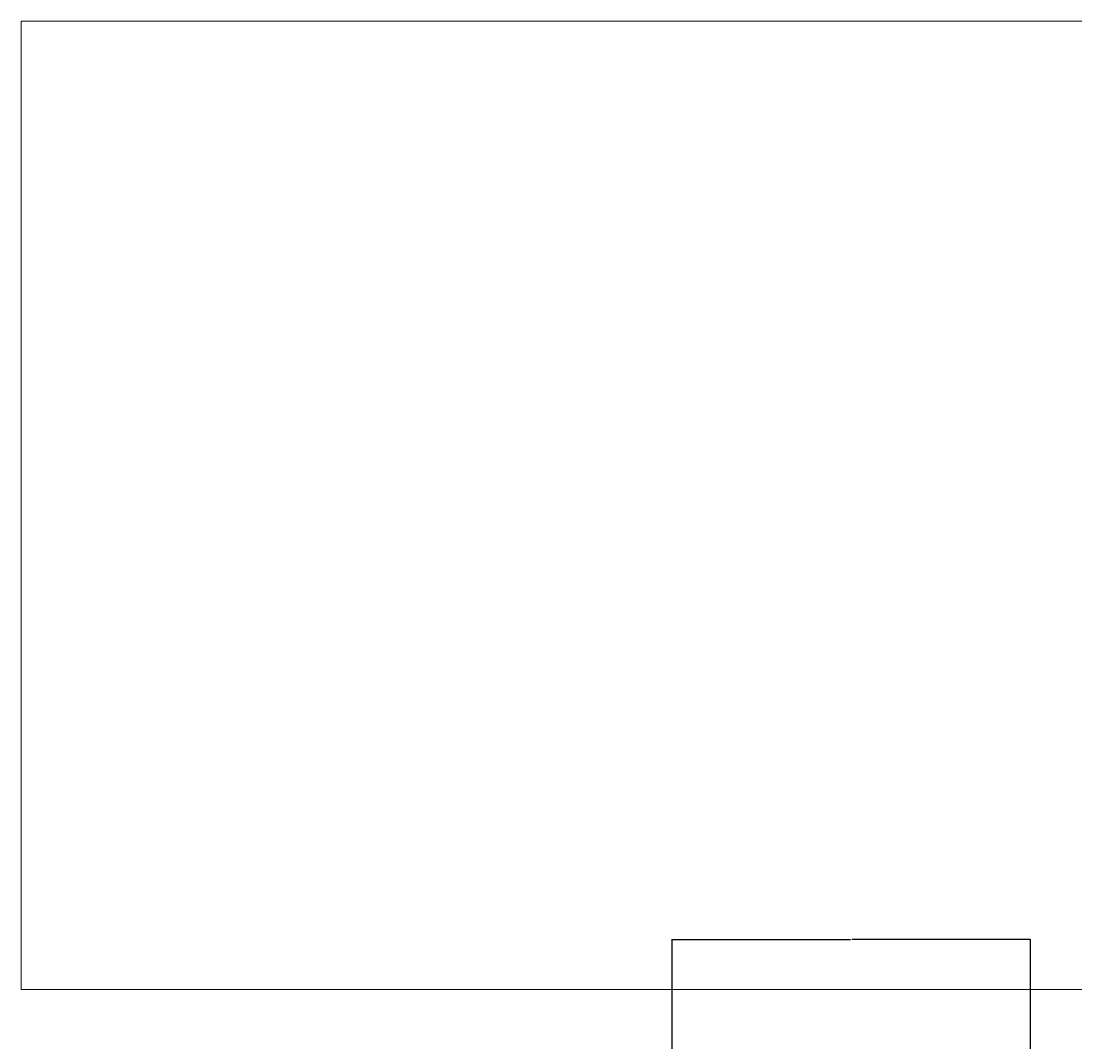
# Model space of a CAD drawing. Units: millimetres. Extents: x 27017497 to 27018854, y 7058029 to 7059154.
# Tile 61 of 91: x 27017710 to 27018246, y 7058634 to 7059154. Entities that reach past the tile are written whole.
import ezdxf

# ---------------------------------------------------------------- set-up
doc = ezdxf.new("R2010")
doc.units = ezdxf.units.MM
doc.layers.add('A-ANNO-DIMS', color=2, linetype='Continuous', lineweight=18)
doc.layers.add('A-ANNO-REFR', color=8, linetype='Continuous', lineweight=13)
doc.styles.get("Standard").update_dxf_attribs({"font": 'arial.ttf'})
doc.dimstyles.get("Standard").update_dxf_attribs({"dimtxt": 0.18, "dimasz": 0.18, "dimexe": 0.18, "dimexo": 0.0625, "dimgap": 0.09, "dimtad": 0, "dimtih": 1, "dimtoh": 1, "dimdec": 4, "dimzin": 0, "dimdsep": 46, "dimtxsty": 'Standard', "dimcen": 0.09, "dimadec": 0, "dimazin": 0, "dimtfac": 1, "dimtdec": 4, "dimtofl": 0, "dimtmove": 0, "dimatfit": 3, "dimfxl": 1, "dimtolj": 1, "dimtzin": 0, "dimarcsym": 0})
picture_1 = doc.add_image_def('image1.png', size_in_pixel=(1340, 653))

# ---------------------------------------------------------------- blocks, each defined once
blk = doc.blocks.new('*D49')
at = {"layer": 'A-ANNO-DIMS', "color": 0, "lineweight": -2, "transparency": 16777216}
for p, q in [((27018041.17, 7058580.97), (27018041.17, 7058686.54)), ((27018041.35, 7058686.36), (27018131.93, 7058686.36)), ((27018223.43, 7058686.36), (27018132.84, 7058686.36)), ((27018223.61, 7058580.97), (27018223.61, 7058686.54))]:
    blk.add_line(p, q, dxfattribs=at)
at = {"layer": 'A-ANNO-DIMS', "color": 0, "transparency": 16777216}
for points in [[(27018041.35, 7058686.39), (27018041.35, 7058686.33), (27018041.17, 7058686.36)], [(27018223.43, 7058686.39), (27018223.43, 7058686.33), (27018223.61, 7058686.36)]]:
    blk.add_solid(points, dxfattribs=at)
at = {"layer": 'Defpoints', "color": 0, "transparency": 16777216}
for p in [(27018223.61, 7058686.36), (27018041.17, 7058580.91), (27018223.61, 7058580.91)]:
    blk.add_point(p, dxfattribs=at)
at = {"layer": 'A-ANNO-DIMS', "color": 0, "transparency": 16777216, "insert": (27018132.39, 7058686.36), "char_height": 0.18, "attachment_point": 5}
blk.add_mtext('\\A1;182.44', dxfattribs=at)

msp = doc.modelspace()

# ---------------------------------------------------------------- dimensions: what is measured, and where the dimension line sits
at = {"layer": 'A-ANNO-DIMS'}
dim = msp.add_linear_dim(base=(27018223.606, 7058686.362), p1=(27018041.166, 7058580.912), p2=(27018223.606, 7058580.912), dimstyle='Standard', override={"dimdec": 2, "dimlfac": 1, "dimrnd": 0, "dimzin": 0, "dimdsep": 46, "dimlunit": 2}, dxfattribs=at)
dim.commit()
dim.dimension.update_dxf_attribs({"geometry": '*D49', "text_midpoint": (27018132.386, 7058686.362)})

# ---------------------------------------------------------------- pictures from other files: only their frames are drawn
at = {"layer": 'A-ANNO-REFR'}
image = msp.add_image(picture_1, insert=(27017709.615, 7058660.772), size_in_units=(1011.788, 493.058), dxfattribs=at)
image.dxf.flags = 7

doc.saveas('drawing.dxf')
